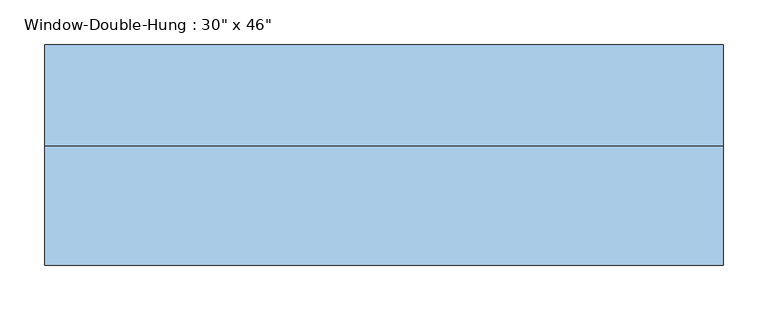
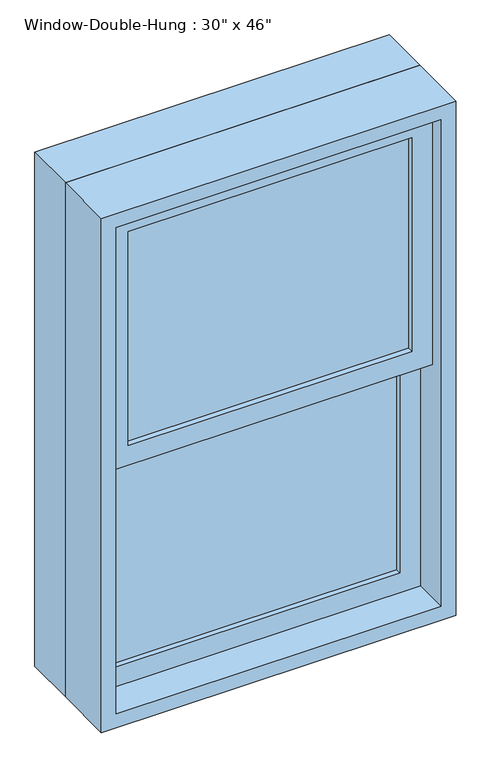
"""IFC4 building model written with IfcOpenShell, lengths in millimetres: window geometry."""

from ifc_helpers import new_model, si_unit, frame, origin, place, context, project, spatial, polyline, outline, extrude, source, transform, mapped, element, save


def window_913990a0(model_context):
    return source(origin(), model_context, "Body", "SweptSolid", [
        extrude(outline(polyline([(304.8, -44.45), (-304.8, -44.45), (-304.8, -38.1), (304.8, -38.1), (304.8, -44.45)])), frame((0.0, 0.0, 990.6), z_axis=(0.0, 0.0, 1.0), x_axis=(1.0, 0.0, 0.0)), (0.0, 0.0, 1.0), 485.775),
        extrude(outline(polyline([(-304.8, -31.75), (-304.8, -25.4), (304.8, -25.4), (304.8, -31.75), (-304.8, -31.75)])), frame((0.0, 0.0, 990.6), z_axis=(0.0, 0.0, 1.0), x_axis=(1.0, 0.0, 0.0)), (0.0, 0.0, 1.0), 485.775),
        extrude(outline(polyline([(304.8, -88.9), (-304.8, -88.9), (-304.8, -82.55), (304.8, -82.55), (304.8, -88.9)])), frame((0.0, 0.0, 1520.825), z_axis=(0.0, 0.0, 1.0), x_axis=(1.0, 0.0, 0.0)), (0.0, 0.0, 1.0), 485.775),
        extrude(outline(polyline([(-304.8, -76.2), (-304.8, -69.85), (304.8, -69.85), (304.8, -76.2), (-304.8, -76.2)])), frame((0.0, 0.0, 1520.825), z_axis=(0.0, 0.0, 1.0), x_axis=(1.0, 0.0, 0.0)), (0.0, 0.0, 1.0), 485.775),
        extrude(outline(polyline([(1520.825, 349.25), (1520.825, -349.25), (946.15, -349.25), (946.15, 349.25), (1520.825, 349.25)]), holes=[polyline([(1476.375, -304.8), (1476.375, 304.8), (990.6, 304.8), (990.6, -304.8), (1476.375, -304.8)])]), frame((0.0, -57.15, 0.0), z_axis=(0.0, 1.0, 0.0), x_axis=(0.0, 0.0, 1.0)), (0.0, 0.0, 1.0), 44.45),
        extrude(outline(polyline([(2051.05, 349.25), (2051.05, -349.25), (1476.375, -349.25), (1476.375, 349.25), (2051.05, 349.25)]), holes=[polyline([(2006.6, -304.8), (2006.6, 304.8), (1520.825, 304.8), (1520.825, -304.8), (2006.6, -304.8)])]), frame((0.0, -101.6, 0.0), z_axis=(0.0, 1.0, 0.0), x_axis=(0.0, 0.0, 1.0)), (0.0, 0.0, 1.0), 44.45),
        extrude(outline(polyline([(2082.8, 381.0), (2082.8, -381.0), (914.4, -381.0), (914.4, 381.0), (2082.8, 381.0)]), holes=[polyline([(2051.05, -349.25), (2051.05, 349.25), (946.15, 349.25), (946.15, -349.25), (2051.05, -349.25)])]), frame((0.0, -133.35, 0.0), z_axis=(0.0, 1.0, 0.0), x_axis=(0.0, 0.0, 1.0)), (0.0, 0.0, 1.0), 133.35),
        extrude(outline(polyline([(2082.8, 381.0), (2082.8, -381.0), (914.4, -381.0), (914.4, 381.0), (2082.8, 381.0)]), holes=[polyline([(2063.75, 361.95), (933.45, 361.95), (933.45, -361.95), (2063.75, -361.95), (2063.75, 361.95)])]), frame((0.0, 0.0, 0.0), z_axis=(0.0, 1.0, 0.0), x_axis=(0.0, 0.0, 1.0)), (0.0, 0.0, 1.0), 114.3),
    ])


if __name__ == "__main__":
    model = new_model("IFC4")
    model_context = context("Model", 3, world=origin())
    ifc_project = project(units=[si_unit("LENGTHUNIT", "METRE", prefix="MILLI")], contexts=[model_context])
    site = spatial("IfcSite", under=ifc_project)
    building = spatial("IfcBuilding", under=site)
    placement = place(None, origin())
    window_shape = window_913990a0(model_context)
    element("IfcWindow", 1, ObjectType="Window-Double-Hung : 30\" x 46\"", at=placement, inside=building, context=model_context, shape_type="MappedRepresentation", body=[
        mapped(window_shape, transform((0.0, 0.0, 0.0), x_axis=(1.0, 0.0, 0.0), y_axis=(0.0, 1.0, 0.0), z_axis=(0.0, 0.0, 1.0))),
    ])
    save(model, "model.ifc")

# Revit data of these elements
# Type "Window-Double-Hung : 30\" x 46\""
#   Type Mark = "13"
#   Fire Rating = "0.5h"
#   Construction Type Id = "DG-DR"
#   Assembly Code = "B2020100"
#   Analytic Construction = "Double glazing - domestic"
#   Wall Thickness [instance default] = 0' - 6"
#   Window Inset [instance default] = 0' - 0"
#   Visual Light Transmittance = 0.81
#   Thermal Resistance (R) = 1.8146 (h·ft²·°F)/BTU
#   Solar Heat Gain Coefficient = 0.76
#   Muntin Width = 2' - 0"
#   Muntin Height = 1' - 7 1/8"
#   Interior Wall Closure [instance default] = 0' - 1 1/2"
#   Rough Width = 2' - 6 1/2"
#   Rough Height = 3' - 10 1/2"
#   Frame Extension [instance default] = 0' - 1 1/4"
#   Exterior Wall Closure [instance default] = 0' - 0 1/2"
#   Extension Jamb [instance default] = 0' - 1 1/2"
#   Heat Transfer Coefficient (U) = 0.5511 BTU/(h·ft²·°F)
#   Height = 3' - 10"
#   Width = 2' - 6"
#   Define Thermal Properties by = 1
#   Top Muntin Visibility = yes
#   Indicator Visibility [instance default] = yes
#   Extension Jamb Visibility [instance default] = yes
#   Interior Trim Visibility [instance default] = yes
#   Exterior Trim Visibility [instance default] = yes
#   Define Thermal Properties by = 1
#   Bottom Muntin Visibility = yes
#   Muntin Pattern = Muntin Pattern_2x2 : Muntin Pattern_2x2
#   Interior Trim Material = Wood - Stained
#   Interior Trim = Trim-Window-Interior-Flat : Picture Frame
#   Exterior Trim Material = Clad - White
#   Exterior Trim = Trim-Window-Exterior-Flat : with Sill
#   Glass Panel Material = Glass
#   Exterior Frame Material = Clad - White
#   Interior Frame Material = Wood - Stained
#   Wall Closure = (empty or 0)
# Element 1 (IfcWindow, "Window-Double-Hung : 30\" x 46\"")
#   Wall Thickness = 0' - 9"
#   Extension Jamb = 0' - 4 1/2"
#   Materials on its faces: "Wood - Stained", "Glass", "Clad - White"
# Materials
#   "Wood - Stained": class "Wood", colour RGB 224 178 126, transparency 0, Cost = 0
#   "Clad - White": class "Wood", colour RGB 242 242 238, transparency 0, Cost = 0
#   "Glass": class "Glass", colour RGB 0 128 192, transparency 0.75, Description = "Soda Lime Glass", Cost = 0
